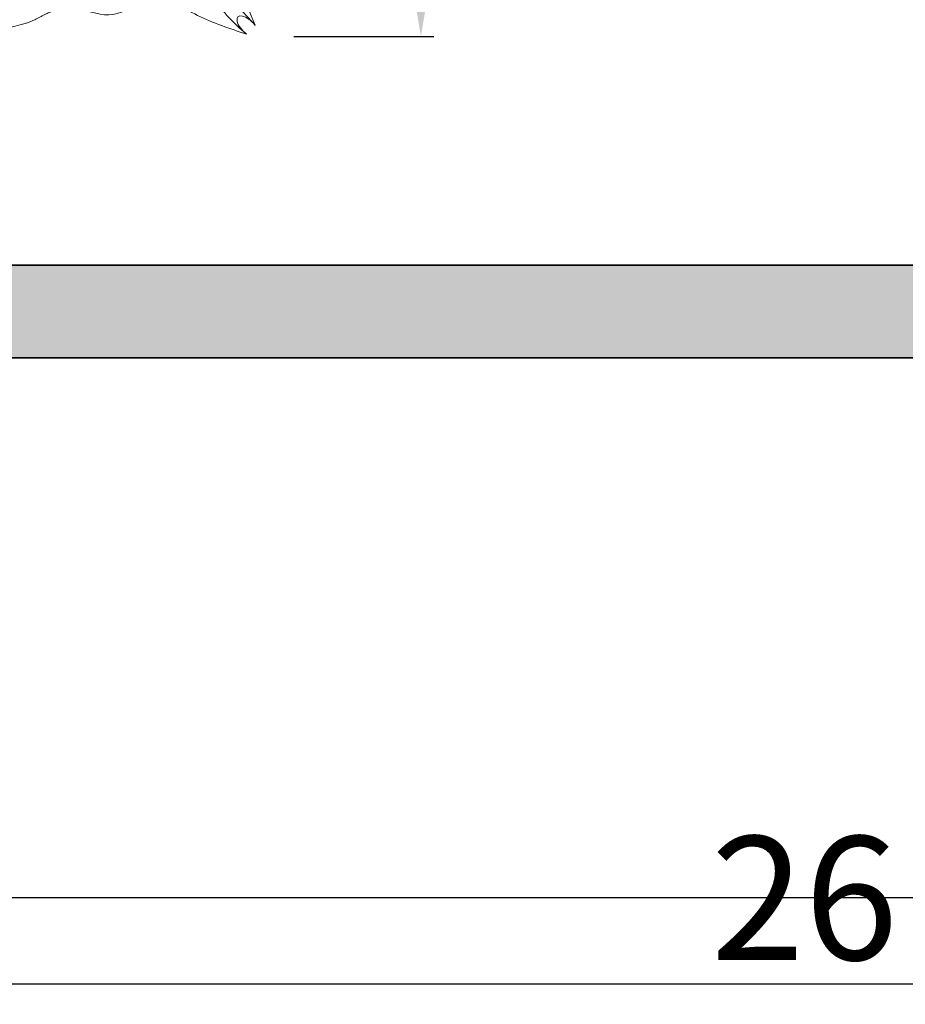
# Model space of a CAD drawing. Units: inches. Extents: x 2083 to 3317, y 1141 to 2115.
# Tile 3 of 256: x 2296 to 2382, y 1201 to 1296. Entities that reach past the tile are written whole.
import ezdxf

# ---------------------------------------------------------------- set-up
doc = ezdxf.new("R2010")
doc.units = ezdxf.units.IN
for name, color, linetype, lineweight in [('A-ANNO-DIMS', 2, 'Continuous', 18), ('A-FURN', 8, 'Continuous', 18), ('A-WALL', 7, 'Continuous', 35), ('www.cadblocksfree.com', 7, 'Continuous', 9)]:
    doc.layers.add(name, color=color, linetype=linetype, lineweight=lineweight)
doc.layers.add('A-WALL-PATT', color=251, linetype='Continuous', lineweight=13, true_color=0x636466)
doc.styles.get("Standard").update_dxf_attribs({"font": 'arial.ttf'})
doc.dimstyles.new('ISO-25', dxfattribs={"dimtxt": 12, "dimasz": 12, "dimexe": 1.25, "dimexo": 0.625, "dimtad": 1, "dimlunit": 3, "dimtxsty": 'Standard', "dimcen": 2.5, "dimadec": 0, "dimazin": 0, "dimtfac": 1, "dimtmove": 0, "dimatfit": 3, "dimfxl": 1, "dimarcsym": 0})

# ---------------------------------------------------------------- blocks, each defined once
blk = doc.blocks.new('bed')
at = {"layer": 'www.cadblocksfree.com', "ltscale": 0.2}
for centre, radius, start, end in [((3370.55, 1414.19), 11.47, 139.4648, 203.3712), ((3367.28, 1412.87), 7.94, 204.0179, 212.619)]:
    blk.add_arc(centre, radius, start, end, dxfattribs=at)
at = {"layer": 'www.cadblocksfree.com', "ltscale": 0.2, "extrusion": (0, 0, -1)}
for centre, major_axis, ratio, start_param, end_param in [((3360.34, 1388.37), (3.04, 3.04), 0.168252, 4.250342, 8.316029), ((3359.29, 1387.32), (1.05, 1.05), 0.453532, 4.422107, 8.144264)]:
    blk.add_ellipse(centre, major_axis=major_axis, ratio=ratio, start_param=start_param, end_param=end_param, dxfattribs=at)
at = {"layer": 'www.cadblocksfree.com', "ltscale": 0.2}
for points, knots in [([(3358.53, 1387.47), (3359.1, 1389.21), (3359.96, 1391.82), (3361.92, 1395.15), (3361.9, 1398.55), (3359.88, 1401.84), (3361.56, 1405.21), (3361.03, 1407.51), (3360.64, 1408.47), (3360.59, 1408.59)], [0, 0, 0, 0, 0.138875, 0.2092702, 0.2901949, 0.3858479, 0.4804923, 0.5489252, 0.5590752, 0.5590752, 0.5590752, 0.5590752]), ([(3430.32, 1386.56), (3427.33, 1387.65), (3422.15, 1389.55), (3414.53, 1384.14), (3405.61, 1387.05), (3396.29, 1386.31), (3386.84, 1381.28), (3377.74, 1390.27), (3370.78, 1384.8), (3364.63, 1383.97), (3363.28, 1388.27), (3360.78, 1387.15), (3359.45, 1386.56)], [0, 0, 0, 0, 8.93042, 15.449194, 25.485629, 34.878505, 43.598887, 54.554403, 64.16647, 67.461673, 70.610457, 74.213583, 74.213583, 74.213583, 74.213583])]:
    blk.add_open_spline(points, degree=3, knots=knots, dxfattribs=at)
blk = doc.blocks.new('*D12')
at = {"layer": 'A-ANNO-DIMS', "color": 0, "lineweight": -2, "transparency": 16777216}
for p, q in [((2226.96, 1262.636), (2226.96, 1201.284)), ((2544.96, 1262.636), (2544.96, 1201.284)), ((2238.96, 1202.534), (2532.96, 1202.534))]:
    blk.add_line(p, q, dxfattribs=at)
at = {"layer": 'A-ANNO-DIMS', "color": 0, "transparency": 16777216}
for points in [[(2238.96, 1204.534), (2238.96, 1200.534), (2226.96, 1202.534)], [(2532.96, 1204.534), (2532.96, 1200.534), (2544.96, 1202.534)]]:
    blk.add_solid(points, dxfattribs=at)
at = {"layer": 'Defpoints', "color": 0, "transparency": 16777216}
for p in [(2226.96, 1263.261), (2544.96, 1263.261), (2544.96, 1202.534)]:
    blk.add_point(p, dxfattribs=at)
at = {"layer": 'A-ANNO-DIMS', "color": 0, "transparency": 16777216, "insert": (2385.96, 1209.286), "char_height": 12, "attachment_point": 5}
blk.add_mtext('26\'-6"', dxfattribs=at)
blk = doc.blocks.new('*D23')
at = {"layer": 'A-ANNO-DIMS', "color": 0, "lineweight": -2, "transparency": 16777216}
for p, q in [((2335.205, 1362.114), (2335.205, 1476.472)), ((2322.885, 1362.114), (2336.455, 1362.114)), ((2335.205, 1306.473), (2335.205, 1350.114)), ((2322.885, 1294.473), (2336.455, 1294.473))]:
    blk.add_line(p, q, dxfattribs=at)
at = {"layer": 'A-ANNO-DIMS', "color": 0, "transparency": 16777216}
for points in [[(2333.205, 1350.114), (2337.205, 1350.114), (2335.205, 1362.114)], [(2333.205, 1306.473), (2337.205, 1306.473), (2335.205, 1294.473)]]:
    blk.add_solid(points, dxfattribs=at)
at = {"layer": 'Defpoints', "color": 0, "transparency": 16777216}
for p in [(2322.26, 1362.114), (2335.205, 1362.114), (2322.26, 1294.473)]:
    blk.add_point(p, dxfattribs=at)
at = {"layer": 'A-ANNO-DIMS', "color": 0, "transparency": 16777216, "insert": (2328.376, 1425.293), "char_height": 12, "attachment_point": 5, "rotation": 90}
blk.add_mtext('5\'-7 1/2" TYP.', dxfattribs=at)
blk = doc.blocks.new('*D34')
at = {"layer": 'A-ANNO-DIMS', "color": 0, "lineweight": -2, "transparency": 16777216}
for p, q in [((2226.96, 1262.636), (2226.96, 1209.661)), ((3126.96, 1262.636), (3126.96, 1209.661)), ((2238.96, 1210.911), (3114.96, 1210.911))]:
    blk.add_line(p, q, dxfattribs=at)
at = {"layer": 'A-ANNO-DIMS', "color": 0, "transparency": 16777216}
for points in [[(2238.96, 1212.911), (2238.96, 1208.911), (2226.96, 1210.911)], [(3114.96, 1212.911), (3114.96, 1208.911), (3126.96, 1210.911)]]:
    blk.add_solid(points, dxfattribs=at)
at = {"layer": 'Defpoints', "color": 0, "transparency": 16777216}
for p in [(2226.96, 1263.261), (3126.96, 1263.261), (3126.96, 1210.911)]:
    blk.add_point(p, dxfattribs=at)
at = {"layer": 'A-ANNO-DIMS', "color": 0, "transparency": 16777216, "insert": (2676.96, 1217.663), "char_height": 12, "attachment_point": 5}
blk.add_mtext('75\'-0"', dxfattribs=at)

msp = doc.modelspace()

# ---------------------------------------------------------------- hatches: boundary and pattern name
at = {"layer": 'A-WALL-PATT'}
h = msp.add_hatch(color=256, dxfattribs=at)
h.dxf.hatch_style = 1
h.paths.add_polyline_path([(3126.96, 2020.761), (2748.96, 2020.761), (2604.96, 2020.761), (2226.96, 2020.761), (2226.96, 1702.761), (2466.96, 1702.761), (2466.96, 1582.761), (2418.96, 1582.761), (2418.96, 1477.761), (2226.96, 1477.761), (2226.96, 1263.261), (2544.96, 1263.261), (2544.96, 1411.761), (2604.96, 1411.761), (2685.96, 1411.761), (2685.96, 1420.761), (2604.96, 1420.761), (2604.96, 1573.761), (2604.96, 1702.761), (2604.96, 2011.761), (2748.96, 2011.761), (2748.96, 1702.761), (2862.96, 1702.761), (2862.96, 1621.761), (2871.96, 1621.761), (2871.96, 1702.761), (2883.96, 1702.761), (2883.96, 1706.939, -0.026459), (2883.96, 1711.761), (2757.96, 1711.761), (2757.96, 1807.761), (2787.96, 1807.761), (2787.96, 1812.261), (2757.96, 1812.261), (2757.96, 2011.761), (2877.96, 2011.761), (2877.96, 1812.261), (2847.96, 1812.261), (2847.96, 1807.761), (2889.836, 1807.761), (2889.836, 1812.261), (2882.46, 1812.261), (2882.46, 2011.761), (3117.96, 2011.761), (3117.96, 1812.261), (2937.836, 1812.261), (2937.836, 1807.761), (2995.71, 1807.761), (2995.71, 1796.118), (3000.21, 1796.118), (3000.21, 1807.761), (3117.96, 1807.761), (3117.96, 1711.761), (3000.21, 1711.761), (3000.21, 1760.118), (2998.573, 1760.118, -0.020711), (2995.71, 1760.118), (2995.71, 1711.761), (2931.96, 1711.761), (2931.96, 1702.761), (3126.96, 1702.761)])
h.paths.add_polyline_path([(2471.46, 2011.761), (2471.46, 1810.011), (2462.717, 1810.011), (2462.717, 1805.511), (2505.96, 1805.511), (2505.96, 1810.011), (2475.96, 1810.011), (2475.96, 2011.761), (2595.96, 2011.761), (2595.96, 1810.011), (2565.96, 1810.011), (2565.96, 1805.511), (2595.96, 1805.511), (2595.96, 1711.761), (2235.96, 1711.761), (2235.96, 1805.511), (2353.71, 1805.511), (2353.71, 1796.054), (2358.21, 1796.054), (2358.21, 1805.511), (2414.717, 1805.511), (2414.717, 1810.011), (2235.96, 1810.011), (2235.96, 2011.761)], flags=16)
h.paths.add_polyline_path([(2270.205, 1994.61), (2270.205, 1970.61), (2246.205, 1970.61), (2246.205, 1994.61)], flags=0)
edge = h.paths.add_edge_path(flags=0)
edge.add_ellipse((2332.027, 1899.798), major_axis=(-3.043, 3.043), ratio=0.168252, start_angle=-161.33217, end_angle=-156.30711, ccw=False)
edge.add_ellipse((2333.082, 1898.744), major_axis=(-1.055, 1.055), ratio=0.453532, start_angle=-123.37102, end_angle=-94.15911)
edge = h.paths.add_edge_path(flags=0)
edge.add_ellipse((2332.027, 1968.876), major_axis=(3.043, 3.043), ratio=0.168252, start_angle=18.66783, end_angle=23.69289)
edge.add_spline(control_points=[(2332.926, 1970.691), (2332.227, 1970.336), (2330.894, 1969.659), (2328.413, 1970.932), (2327.204, 1967.749), (2324.71, 1969.956), (2322.533, 1967.012), (2320.013, 1971.296), (2317.68, 1968.158), (2316.041, 1967.102), (2315.427, 1966.81)], knot_values=[0, 0, 0, 0, 2.267059, 4.324559, 6.685584, 8.878641, 11.121502, 14.300359, 17.755284, 19.732645, 19.732645, 19.732645, 19.732645], degree=3, periodic=0)
edge.add_ellipse((2332.027, 1968.876), major_axis=(3.043, 3.043), ratio=0.168252, start_angle=18.66783, end_angle=23.69289, ccw=False)
edge.add_ellipse((2333.082, 1969.931), major_axis=(1.055, 1.055), ratio=0.453532, start_angle=56.62898, end_angle=85.84089, ccw=False)
edge = h.paths.add_edge_path(flags=0)
edge.add_spline(control_points=[(2296.428, 1967.988), (2293.628, 1965.336), (2287.704, 1959.727), (2299.744, 1949.996), (2294.533, 1935.669), (2290.573, 1920.604), (2293.394, 1909.974), (2296.185, 1904.967)], knot_values=[0.099185, 0.099185, 0.099185, 0.099185, 0.345301, 0.619822, 0.982653, 1.386093, 1.810555, 1.810555, 1.810555, 1.810555], degree=3, periodic=0)
edge.add_spline(control_points=[(2296.185, 1904.967), (2297.384, 1902.619), (2298.001, 1901.949), (2298.553, 1901.468)], knot_values=[0.006246, 0.006246, 0.006246, 0.006246, 0.055476, 0.055476, 0.055476, 0.055476], degree=3, periodic=0)
edge.add_spline(control_points=[(2298.553, 1901.468), (2297.259, 1900.923), (2295.225, 1900.232), (2293.06, 1900.614), (2292.101, 1900.788), (2292.09, 1900.791)], knot_values=[0.312835, 0.312835, 0.312835, 0.312835, 0.40178, 0.474987, 0.475903, 0.475903, 0.475903, 0.475903], degree=3, periodic=0)
edge.add_arc((2292.794, 1904.664), 3.937, 215.4209, 259.69818, ccw=False)
edge.add_spline(control_points=[(2289.585, 1902.382), (2289.477, 1902.535), (2289.368, 1902.688), (2289.261, 1902.841)], knot_values=[0.102872, 0.102872, 0.102872, 0.102872, 0.116896, 0.116896, 0.116896, 0.116896], degree=3, periodic=0)
edge.add_spline(control_points=[(2289.261, 1902.841), (2288.687, 1902.55), (2287.64, 1902.02), (2285.881, 1901.874), (2283.853, 1901.504), (2281.72, 1899.711), (2278.467, 1899.493), (2276.157, 1901.883), (2272.259, 1899.804), (2267.778, 1901.843), (2262.244, 1900.184), (2257.415, 1901.782), (2254.318, 1900.726), (2253.178, 1900.337)], knot_values=[0, 0, 0, 0, 1.907977, 3.477176, 5.261074, 7.972851, 11.680248, 13.717921, 16.939592, 22.789562, 27.502503, 33.595215, 37.145618, 37.145618, 37.145618, 37.145618], degree=3, periodic=0)
edge.add_line((2253.178, 1900.337), (2250.244, 1902.841))
edge.add_line((2250.244, 1902.841), (2250.244, 1965.833))
edge.add_line((2250.244, 1965.833), (2253.178, 1968.337))
edge.add_spline(control_points=[(2253.178, 1968.337), (2254.318, 1967.948), (2257.415, 1966.892), (2262.244, 1968.49), (2267.778, 1966.831), (2271.527, 1968.537), (2273.876, 1967.828), (2274.207, 1967.728)], knot_values=[0, 0, 0, 0, 0.09018, 0.244935, 0.364644, 0.513233, 0.537855, 0.537855, 0.537855, 0.537855], degree=3, periodic=0)
edge.add_arc((2274.353, 1963.793), 3.937, 72.05113, 92.12795, ccw=False)
edge.add_arc((2281.297, 1985.23), 18.596, 252.05113, 288.56572)
edge.add_arc((2292.317, 1956.029), 12.646, 71.02679, 113.77822, ccw=False)
edge = h.paths.add_edge_path(flags=0)
edge.add_spline(control_points=[(2274.899, 1951.856), (2275.066, 1951.617), (2275.233, 1951.377), (2275.398, 1951.136)], knot_values=[1.409916, 1.409916, 1.409916, 1.409916, 1.43159, 1.43159, 1.43159, 1.43159], degree=3, periodic=0)
edge.add_spline(control_points=[(2275.398, 1951.136), (2275.792, 1950.562), (2276.179, 1949.984), (2276.546, 1949.397)], knot_values=[1.358238, 1.358238, 1.358238, 1.358238, 1.409916, 1.409916, 1.409916, 1.409916], degree=3, periodic=0)
edge.add_line((2276.546, 1949.397), (2277.437, 1947.862))
edge.add_spline(control_points=[(2277.437, 1947.862), (2276.304, 1945.673), (2274.64, 1942.427), (2274.632, 1938.094), (2272.799, 1930.852), (2274.356, 1943.897), (2275.948, 1947.923), (2276.546, 1949.397)], knot_values=[0.005632, 0.005632, 0.005632, 0.005632, 0.186014, 0.266002, 0.357087, 0.59639, 0.739732, 0.739732, 0.739732, 0.739732], degree=3, periodic=0)
edge.add_spline(control_points=[(2276.546, 1949.397), (2276.179, 1949.984), (2275.792, 1950.562), (2275.398, 1951.136)], knot_values=[1.358238, 1.358238, 1.358238, 1.358238, 1.409916, 1.409916, 1.409916, 1.409916], degree=3, periodic=0)
edge.add_spline(control_points=[(2275.398, 1951.136), (2274.943, 1950.08), (2274.208, 1948.025), (2273.935, 1944.851), (2272.469, 1937.627), (2273.466, 1945.696), (2274.701, 1951.059), (2274.899, 1951.856)], knot_values=[0.104364, 0.104364, 0.104364, 0.104364, 0.189636, 0.269624, 0.36071, 0.600013, 0.644622, 0.644622, 0.644622, 0.644622], degree=3, periodic=0)
h.paths.add_polyline_path([(2269.168, 1963.128, -0.357527), (2268.171, 1960.976, -0.092561), (2268.171, 1939.436, -0.357527), (2269.168, 1937.285, -0.357527), (2267.016, 1938.282, -0.164785), (2254.686, 1938.282, -0.357527), (2252.534, 1937.285, -0.357527), (2253.531, 1939.436, -0.092561), (2253.531, 1960.976, -0.357527), (2252.534, 1963.128, -0.357527), (2254.686, 1962.131, -0.164785), (2267.016, 1962.131, -0.357527)], flags=0)
h.paths.add_polyline_path([(2248.874, 1967.802), (2248.874, 1957.028), (2249.458, 1957.028), (2249.458, 1911.647), (2248.874, 1911.647), (2248.874, 1900.873), (2246.512, 1900.873, 0.197327), (2244.15, 1902.457), (2244.15, 1966.218, 0.197327), (2246.512, 1967.802)], flags=0)
h.paths.add_polyline_path([(2269.168, 1931.389, -0.357527), (2268.171, 1929.238, -0.092561), (2268.171, 1907.698, -0.357527), (2269.168, 1905.547, -0.357527), (2267.016, 1906.544, -0.164785), (2254.686, 1906.544, -0.357527), (2252.534, 1905.547, -0.357527), (2253.531, 1907.698, -0.092561), (2253.531, 1929.238, -0.357527), (2252.534, 1931.389, -0.357527), (2254.686, 1930.392, -0.164785), (2267.016, 1930.392, -0.357527)], flags=0)
edge = h.paths.add_edge_path(flags=0)
edge.add_spline(control_points=[(2276.197, 1906.724), (2276.168, 1909.029), (2276.114, 1913.372), (2270.598, 1924.925), (2273.905, 1919.013), (2275.922, 1916.262), (2275.475, 1912.402), (2277.258, 1910.381), (2276.696, 1908.225), (2276.646, 1906.813), (2276.618, 1906.008)], knot_values=[0, 0, 0, 0, 8.61026, 16.221274, 18.843057, 23.804898, 27.440828, 29.356102, 31.203478, 33.650687, 33.650687, 33.650687, 33.650687], degree=3, periodic=0)
edge.add_spline(control_points=[(2276.618, 1906.008), (2276.623, 1905.624), (2276.498, 1904.629), (2275.442, 1903.855), (2274.937, 1903.08), (2274.859, 1902.841)], knot_values=[0.156488, 0.156488, 0.156488, 0.156488, 0.184398, 0.231376, 0.250598, 0.250598, 0.250598, 0.250598], degree=3, periodic=0)
edge.add_line((2274.859, 1902.841), (2276.506, 1902.841))
edge.add_spline(control_points=[(2276.506, 1902.841), (2276.788, 1903.085), (2277.665, 1904.125), (2278.25, 1904.341), (2277.654, 1908.527), (2278.156, 1906.228), (2278.1, 1905.286), (2278.847, 1904.069), (2277.857, 1903.415), (2277.874, 1902.991), (2277.904, 1902.841)], knot_values=[0.059574, 0.059574, 0.059574, 0.059574, 0.080753, 0.103741, 0.16972, 0.176036, 0.207137, 0.240474, 0.262341, 0.27366, 0.27366, 0.27366, 0.27366], degree=3, periodic=0)
edge.add_line((2277.904, 1902.841), (2280.03, 1902.841))
edge.add_spline(control_points=[(2280.03, 1902.841), (2279.888, 1903.088), (2279.499, 1903.982), (2280.152, 1905.939), (2278.104, 1909.658), (2279.762, 1907.185), (2280.328, 1904.875), (2280.485, 1903.49), (2281.463, 1903.249), (2281.758, 1902.936), (2281.834, 1902.841)], knot_values=[0.013856, 0.013856, 0.013856, 0.013856, 0.034874, 0.088867, 0.107879, 0.126738, 0.158714, 0.193757, 0.217487, 0.226722, 0.226722, 0.226722, 0.226722], degree=3, periodic=0)
edge.add_spline(control_points=[(2281.834, 1902.841), (2281.788, 1902.827), (2281.647, 1902.783), (2281.396, 1902.859), (2281.088, 1902.985), (2280.721, 1903.061), (2280.333, 1903.026), (2280.125, 1902.899), (2280.03, 1902.841)], knot_values=[0, 0, 0, 0, 0.14413, 0.435517, 0.749276, 1.153046, 1.548371, 1.878348, 1.878348, 1.878348, 1.878348], degree=3, periodic=0)
edge.add_line((2280.03, 1902.841), (2277.904, 1902.841))
edge.add_spline(control_points=[(2277.904, 1902.841), (2277.893, 1902.796), (2277.865, 1902.68), (2277.607, 1902.687), (2277.274, 1902.801), (2276.838, 1902.62), (2276.584, 1902.789), (2276.506, 1902.841)], knot_values=[0, 0, 0, 0, 0.127189, 0.326199, 0.628009, 1.24357, 1.515331, 1.515331, 1.515331, 1.515331], degree=3, periodic=0)
edge.add_line((2276.506, 1902.841), (2274.859, 1902.841))
edge.add_spline(control_points=[(2274.859, 1902.841), (2274.814, 1902.899), (2274.725, 1903.013), (2274.493, 1903.119), (2274.244, 1902.961), (2273.937, 1903.185), (2273.614, 1902.983), (2273.408, 1902.883), (2273.322, 1902.841)], knot_values=[0, 0, 0, 0, 0.21843, 0.436957, 0.687977, 0.990379, 1.398396, 1.69185, 1.69185, 1.69185, 1.69185], degree=3, periodic=0)
edge.add_spline(control_points=[(2273.322, 1902.841), (2273.617, 1903.446), (2274.274, 1904.538), (2276.027, 1904.574), (2276.207, 1906.584), (2276.197, 1906.724)], knot_values=[0.012227, 0.012227, 0.012227, 0.012227, 0.059472, 0.106218, 0.134458, 0.134458, 0.134458, 0.134458], degree=3, periodic=0)
h.paths.add_polyline_path([(2270.776, 1897.79), (2270.776, 1873.79), (2246.776, 1873.79), (2246.776, 1897.79)], flags=0)
h.paths.add_polyline_path([(2353.71, 1760.005), (2353.71, 1760.054), (2358.21, 1760.054, -0.033729)], flags=0)
h.paths.add_polyline_path([(2321.819, 1737.529), (2341.995, 1737.529, -0.414214), (2343.203, 1736.321), (2343.203, 1721.021, -0.414214), (2341.995, 1719.813), (2321.819, 1719.813, -0.414214), (2320.611, 1721.021), (2320.611, 1736.321, -0.414214)], flags=0)
h.paths.add_polyline_path([(2324.235, 1736.321), (2339.579, 1736.321, -0.414214), (2341.995, 1733.905), (2341.995, 1725.45, -0.414214), (2339.579, 1723.034), (2333.681, 1723.034), (2333.845, 1722.045, -0.870646), (2335.425, 1721.826, -0.767327), (2333.923, 1721.423), (2331.291, 1721.423, -0.767327), (2329.788, 1721.826, -0.870646), (2331.368, 1722.045), (2331.533, 1723.034), (2324.235, 1723.034, -0.414214), (2321.819, 1725.45), (2321.819, 1733.905, -0.414214)], flags=0)
h.paths.add_polyline_path([(2570.484, 1928.615), (2589.684, 1928.615), (2590.169, 1928.615), (2590.169, 1904.993), (2570.484, 1904.993)], flags=0)
h.paths.add_polyline_path([(2574.447, 1927.264, -1), (2572.829, 1927.264, -1)], flags=0)
h.paths.add_polyline_path([(2573.09, 1926.941), (2573.925, 1927.776), (2574.148, 1927.553), (2573.313, 1926.718)], flags=0)
h.paths.add_polyline_path([(2578.779, 1919.73, -1), (2571.592, 1919.73, -1)], flags=0)
h.paths.add_polyline_path([(2578.385, 1919.73, -1), (2571.985, 1919.73, -1)], flags=0)
h.paths.add_polyline_path([(2331.596, 1729.476, -1), (2333.618, 1729.476, -1)], flags=0)
h.paths.add_polyline_path([(2578.034, 1927.264, -1), (2576.416, 1927.264, -1)], flags=0)
h.paths.add_polyline_path([(2576.689, 1927.531), (2576.912, 1927.754), (2577.747, 1926.919), (2577.524, 1926.696)], flags=0)
h.paths.add_polyline_path([(2578.139, 1909.86, -1), (2572.232, 1909.86, -1)], flags=0)
h.paths.add_polyline_path([(2577.745, 1909.86, -1), (2572.625, 1909.86, -1)], flags=0)
h.paths.add_polyline_path([(2583.798, 1927.264, -1), (2582.179, 1927.264, -1)], flags=0)
h.paths.add_polyline_path([(2582.719, 1927.754), (2583.554, 1926.919), (2583.331, 1926.696), (2582.496, 1927.531)], flags=0)
h.paths.add_polyline_path([(2582.496, 1927.531), (2582.719, 1927.754), (2583.554, 1926.919), (2583.331, 1926.696)], flags=0)
h.paths.add_polyline_path([(2587.739, 1920.53, -1), (2581.832, 1920.53, -1)], flags=0)
h.paths.add_polyline_path([(2587.345, 1920.53, -1), (2582.225, 1920.53, -1)], flags=0)
h.paths.add_polyline_path([(2587.385, 1927.264, -1), (2585.766, 1927.264, -1)], flags=0)
h.paths.add_polyline_path([(2586.082, 1926.98), (2586.917, 1927.815), (2587.14, 1927.593), (2586.305, 1926.758)], flags=0)
h.paths.add_polyline_path([(2588.379, 1910.66, -1), (2581.192, 1910.66, -1)], flags=0)
h.paths.add_polyline_path([(2587.985, 1910.66, -1), (2581.585, 1910.66, -1)], flags=0)
h.paths.add_polyline_path([(2417.168, 1729.478), (2437.344, 1729.478, -0.414214), (2438.552, 1728.27), (2438.552, 1712.969, -0.414214), (2437.344, 1711.761), (2417.168, 1711.761, -0.414214), (2415.96, 1712.969), (2415.96, 1728.27, -0.414214)], flags=0)
h.paths.add_polyline_path([(2419.584, 1728.27), (2434.928, 1728.27, -0.414214), (2437.344, 1725.854), (2437.344, 1717.398, -0.414214), (2434.928, 1714.983), (2429.029, 1714.983), (2429.194, 1713.994, -0.870646), (2430.774, 1713.775, -0.767327), (2429.271, 1713.372), (2426.64, 1713.372, -0.767327), (2425.137, 1713.775, -0.870646), (2426.717, 1713.994), (2426.882, 1714.983), (2419.584, 1714.983, -0.414214), (2417.168, 1717.398), (2417.168, 1725.854, -0.414214)], flags=0)
h.paths.add_polyline_path([(2419.584, 1728.27), (2434.928, 1728.27, -0.414214), (2437.344, 1725.854), (2437.344, 1717.398, -0.414214), (2434.928, 1714.983), (2429.029, 1714.983), (2428.358, 1719.009), (2427.553, 1719.009), (2426.882, 1714.983), (2419.584, 1714.983, -0.414214), (2417.168, 1717.398), (2417.168, 1725.854, -0.414214)], flags=0)
h.paths.add_polyline_path([(2426.944, 1721.425, -1), (2428.967, 1721.425, -1)], flags=0)
h.paths.add_polyline_path([(2475.96, 1702.761), (2595.96, 1702.761), (2595.96, 1582.761), (2475.96, 1582.761)], flags=16)
h.paths.add_polyline_path([(2427.96, 1573.761), (2595.96, 1573.761), (2595.96, 1468.761), (2595.96, 1420.761), (2384.46, 1420.761), (2384.46, 1468.761), (2427.96, 1468.761)], flags=16)
h.paths.add_polyline_path([(2379.96, 1468.761), (2379.96, 1420.761), (2235.96, 1420.761), (2235.96, 1468.761)], flags=16)
h.paths.add_polyline_path([(2317.816, 1466.696), (2337.992, 1466.696, -0.414214), (2339.2, 1465.488), (2339.2, 1450.187, -0.414214), (2337.992, 1448.979), (2317.816, 1448.979, -0.414214), (2316.608, 1450.187), (2316.608, 1465.488, -0.414214)], flags=0)
h.paths.add_polyline_path([(2320.232, 1465.488), (2335.576, 1465.488, -0.414214), (2337.992, 1463.072), (2337.992, 1454.616, -0.414214), (2335.576, 1452.2), (2329.677, 1452.2), (2329.842, 1451.212, -0.870646), (2331.422, 1450.992, -0.767327), (2329.92, 1450.59), (2327.288, 1450.59, -0.767327), (2325.785, 1450.992, -0.870646), (2327.365, 1451.212), (2327.53, 1452.2), (2320.232, 1452.2, -0.414214), (2317.816, 1454.616), (2317.816, 1463.072, -0.414214)], flags=0)
h.paths.add_polyline_path([(2320.232, 1465.488), (2335.576, 1465.488, -0.414214), (2337.992, 1463.072), (2337.992, 1454.616, -0.414214), (2335.576, 1452.2), (2329.677, 1452.2), (2329.006, 1456.227), (2328.201, 1456.227), (2327.53, 1452.2), (2320.232, 1452.2, -0.414214), (2317.816, 1454.616), (2317.816, 1463.072, -0.414214)], flags=0)
h.paths.add_polyline_path([(2327.593, 1458.643, -1), (2329.615, 1458.643, -1)], flags=0)
h.paths.add_polyline_path([(2244.412, 1433.34), (2241.921, 1433.34, -0.414214), (2240.018, 1435.244), (2240.018, 1440.953, -0.414211), (2241.921, 1442.856), (2244.412, 1442.856, -1.976472)], flags=0)
h.paths.add_polyline_path([(2245.357, 1434.398, -0.414214), (2245.357, 1441.799, -2.144098)], flags=0)
h.paths.add_polyline_path([(2535.96, 1416.261), (2535.96, 1272.261), (2235.96, 1272.261), (2235.96, 1416.261)], flags=16)
h.paths.add_polyline_path([(2260.12, 1384.293), (2260.12, 1362.039), (2237.865, 1362.039), (2237.865, 1384.293)], flags=0)
edge = h.paths.add_edge_path(flags=0)
edge.add_line((2318.252, 1362.093), (2318.146, 1362.001))
edge.add_ellipse((2317.445, 1360.431), major_axis=(2.822, 2.822), ratio=0.168252, start_angle=18.66783, end_angle=20.94813, ccw=False)
edge.add_ellipse((2318.423, 1361.409), major_axis=(0.978, 0.978), ratio=0.453532, start_angle=56.62898, end_angle=70.2262, ccw=False)
edge = h.paths.add_edge_path(flags=0)
edge.add_line((2319.107, 1295.571), (2319.015, 1295.677))
edge.add_ellipse((2317.445, 1296.378), major_axis=(-2.822, 2.822), ratio=0.168252, start_angle=-161.33217, end_angle=-159.05187, ccw=False)
edge.add_ellipse((2318.423, 1295.4), major_axis=(-0.978, 0.978), ratio=0.453532, start_angle=-123.37102, end_angle=-109.7738)
edge = h.paths.add_edge_path(flags=0)
edge.add_spline(control_points=[(2284.21, 1301.17), (2284.581, 1300.445), (2284.891, 1299.892), (2285.16, 1299.461)], knot_values=[0.039066, 0.039066, 0.039066, 0.039066, 0.055476, 0.055476, 0.055476, 0.055476], degree=3, periodic=0)
edge.add_line((2285.16, 1299.461), (2284.21, 1301.17))
edge = h.paths.add_edge_path(flags=0)
edge.add_line((2280.412, 1297.298), (2283.37, 1297.036))
edge.add_line((2283.37, 1297.036), (2286.406, 1297.926))
edge.add_spline(control_points=[(2286.406, 1297.926), (2285.305, 1297.463), (2284.345, 1297.129), (2283.37, 1297.036)], knot_values=[0.394369, 0.394369, 0.394369, 0.394369, 0.475903, 0.475903, 0.475903, 0.475903], degree=3, periodic=0)
edge.add_spline(control_points=[(2283.37, 1297.036), (2283.281, 1297.028), (2282.316, 1296.957), (2281.313, 1297.134), (2280.423, 1297.296), (2280.412, 1297.298)], knot_values=[0.312835, 0.312835, 0.312835, 0.312835, 0.320246, 0.393453, 0.394369, 0.394369, 0.394369, 0.394369], degree=3, periodic=0)
edge = h.paths.add_edge_path(flags=0)
edge.add_line((2284.436, 1359.607), (2280.446, 1355.328))
edge.add_line((2280.446, 1355.328), (2279.58, 1351.018))
edge.add_line((2279.58, 1351.018), (2282.413, 1346.58))
edge.add_spline(control_points=[(2282.413, 1346.58), (2283.153, 1345.589), (2284.253, 1344.029), (2284.801, 1342.387), (2284.935, 1341.806)], knot_values=[1.240098, 1.240098, 1.240098, 1.240098, 1.332892, 1.382712, 1.382712, 1.382712, 1.382712], degree=3, periodic=0)
edge.add_spline(control_points=[(2284.935, 1341.806), (2285.319, 1340.141), (2285.233, 1338.409), (2284.91, 1336.654)], knot_values=[1.097484, 1.097484, 1.097484, 1.097484, 1.240098, 1.240098, 1.240098, 1.240098], degree=3, periodic=0)
edge.add_spline(control_points=[(2284.91, 1336.654), (2284.587, 1334.899), (2284.027, 1333.12), (2283.463, 1331.361)], knot_values=[0.95487, 0.95487, 0.95487, 0.95487, 1.097484, 1.097484, 1.097484, 1.097484], degree=3, periodic=0)
edge.add_line((2283.463, 1331.361), (2281.89, 1326.153))
edge.add_line((2281.89, 1326.153), (2280.756, 1321.056))
edge.add_line((2280.756, 1321.056), (2280.299, 1316.002))
edge.add_line((2280.299, 1316.002), (2280.716, 1310.95))
edge.add_line((2280.716, 1310.95), (2282.028, 1305.972))
edge.add_line((2282.028, 1305.972), (2284.21, 1301.17))
edge.add_spline(control_points=[(2284.21, 1301.17), (2283.341, 1302.73), (2282.612, 1304.336), (2282.028, 1305.972)], knot_values=[0.099185, 0.099185, 0.099185, 0.099185, 0.241799, 0.241799, 0.241799, 0.241799], degree=3, periodic=0)
edge.add_spline(control_points=[(2282.028, 1305.972), (2281.444, 1307.608), (2281.005, 1309.273), (2280.716, 1310.95)], knot_values=[0.241799, 0.241799, 0.241799, 0.241799, 0.384413, 0.384413, 0.384413, 0.384413], degree=3, periodic=0)
edge.add_spline(control_points=[(2280.716, 1310.95), (2280.433, 1312.588), (2280.289, 1314.277), (2280.299, 1315.962), (2280.299, 1316.002)], knot_values=[0.384413, 0.384413, 0.384413, 0.384413, 0.523647, 0.527028, 0.527028, 0.527028, 0.527028], degree=3, periodic=0)
edge.add_spline(control_points=[(2280.299, 1316.002), (2280.312, 1317.687), (2280.478, 1319.368), (2280.756, 1321.056)], knot_values=[0.527028, 0.527028, 0.527028, 0.527028, 0.669642, 0.669642, 0.669642, 0.669642], degree=3, periodic=0)
edge.add_spline(control_points=[(2280.756, 1321.056), (2281.035, 1322.744), (2281.426, 1324.44), (2281.89, 1326.153)], knot_values=[0.669642, 0.669642, 0.669642, 0.669642, 0.812256, 0.812256, 0.812256, 0.812256], degree=3, periodic=0)
edge.add_spline(control_points=[(2281.89, 1326.153), (2282.264, 1327.533), (2282.788, 1329.262), (2283.353, 1331.018), (2283.463, 1331.361)], knot_values=[0.812256, 0.812256, 0.812256, 0.812256, 0.927087, 0.95487, 0.95487, 0.95487, 0.95487], degree=3, periodic=0)
edge.add_line((2283.463, 1331.361), (2284.91, 1336.654))
edge.add_line((2284.91, 1336.654), (2284.935, 1341.806))
edge.add_line((2284.935, 1341.806), (2282.413, 1346.58))
edge.add_spline(control_points=[(2282.413, 1346.58), (2281.275, 1348.104), (2280.078, 1349.57), (2279.58, 1351.018)], knot_values=[1.382712, 1.382712, 1.382712, 1.382712, 1.525326, 1.525326, 1.525326, 1.525326], degree=3, periodic=0)
edge.add_spline(control_points=[(2279.58, 1351.018), (2279.443, 1351.415), (2279.136, 1352.857), (2279.735, 1354.29), (2280.446, 1355.328)], knot_values=[1.525326, 1.525326, 1.525326, 1.525326, 1.564439, 1.667941, 1.667941, 1.667941, 1.667941], degree=3, periodic=0)
edge.add_spline(control_points=[(2280.446, 1355.328), (2281.426, 1356.758), (2282.931, 1358.183), (2284.436, 1359.607)], knot_values=[1.667941, 1.667941, 1.667941, 1.667941, 1.810555, 1.810555, 1.810555, 1.810555], degree=3, periodic=0)
edge.add_arc((2280.623, 1348.518), 11.726, 71.02679, 113.77822)
edge.add_arc((2270.405, 1375.595), 17.244, 252.05113, 288.56572, ccw=False)
edge.add_arc((2263.966, 1355.718), 3.651, 72.05113, 92.12795)
edge.add_arc((2263.966, 1355.718), 3.651, 92.12795, 177.98513)
edge.add_spline(control_points=[(2260.318, 1355.846), (2260.26, 1354.221), (2260.551, 1350.187), (2262.999, 1346.766), (2264.473, 1344.649)], knot_values=[1.43159, 1.43159, 1.43159, 1.43159, 1.564144, 1.770695, 1.770695, 1.770695, 1.770695], degree=3, periodic=0)
edge.add_line((2264.473, 1344.649), (2264.936, 1343.983))
edge.add_spline(control_points=[(2263.801, 1340.248), (2263.843, 1340.514), (2264.067, 1341.756), (2264.513, 1343.002), (2264.935, 1343.981)], knot_values=[0.53657, 0.53657, 0.53657, 0.53657, 0.559349, 0.644622, 0.644622, 0.644622, 0.644622], degree=3, periodic=0)
edge.add_spline(control_points=[(2264.935, 1343.981), (2265.118, 1343.715), (2265.299, 1343.448), (2265.477, 1343.179)], knot_values=[1.384077, 1.384077, 1.384077, 1.384077, 1.409916, 1.409916, 1.409916, 1.409916], degree=3, periodic=0)
edge.add_spline(control_points=[(2265.477, 1343.179), (2265.655, 1342.911), (2265.829, 1342.641), (2265.999, 1342.369)], knot_values=[1.358238, 1.358238, 1.358238, 1.358238, 1.384077, 1.384077, 1.384077, 1.384077], degree=3, periodic=0)
edge.add_line((2265.999, 1342.369), (2266.826, 1340.946))
edge.add_spline(control_points=[(2266.826, 1340.946), (2268.894, 1337.09), (2271.398, 1325.843), (2270.516, 1310.569), (2275.919, 1301.861), (2277.79, 1299.199)], knot_values=[0.116896, 0.116896, 0.116896, 0.116896, 0.472987, 1.050969, 1.313793, 1.313793, 1.313793, 1.313793], degree=3, periodic=0)
edge.add_spline(control_points=[(2277.79, 1299.199), (2277.839, 1299.128), (2277.889, 1299.057), (2277.94, 1298.987)], knot_values=[0.109884, 0.109884, 0.109884, 0.109884, 0.116896, 0.116896, 0.116896, 0.116896], degree=3, periodic=0)
edge.add_line((2277.94, 1298.987), (2277.789, 1299.199))
edge.add_spline(control_points=[(2277.789, 1299.199), (2277.257, 1298.929), (2276.286, 1298.438), (2275.039, 1298.334), (2274.383, 1298.239), (2274.215, 1298.209)], knot_values=[33.12187, 33.12187, 33.12187, 33.12187, 35.029056, 36.598255, 37.144827, 37.144827, 37.144827, 37.144827], degree=3, periodic=0)
edge.add_line((2274.215, 1298.209), (2273.073, 1297.893))
edge.add_spline(control_points=[(2273.073, 1297.893), (2272.323, 1297.58), (2271.039, 1296.511), (2269.248, 1296.226), (2268.423, 1296.375)], knot_values=[26.532584, 26.532584, 26.532584, 26.532584, 29.198919, 31.839101, 31.839101, 31.839101, 31.839101], degree=3, periodic=0)
edge.add_line((2268.423, 1296.375), (2263.879, 1297.458))
edge.add_spline(control_points=[(2263.879, 1297.458), (2263.556, 1297.359), (2261.86, 1296.839), (2260.239, 1297.282), (2258.933, 1297.516)], knot_values=[15.919551, 15.919551, 15.919551, 15.919551, 16.939592, 21.226067, 21.226067, 21.226067, 21.226067], degree=3, periodic=0)
edge.add_line((2258.933, 1297.516), (2254.055, 1297.329))
edge.add_spline(control_points=[(2254.055, 1297.329), (2253.756, 1297.296), (2252.114, 1297.165), (2250.462, 1297.544), (2249.13, 1297.668)], knot_values=[5.306517, 5.306517, 5.306517, 5.306517, 6.276435, 10.613034, 10.613034, 10.613034, 10.613034], degree=3, periodic=0)
edge.add_line((2249.13, 1297.668), (2244.332, 1296.878))
edge.add_line((2244.332, 1296.878), (2241.611, 1299.199))
edge.add_line((2241.611, 1299.199), (2241.611, 1357.609))
edge.add_line((2241.611, 1357.609), (2244.332, 1359.931))
edge.add_line((2244.332, 1359.931), (2252.729, 1359.543))
edge.add_spline(control_points=[(2252.729, 1359.543), (2252.871, 1359.546), (2253.306, 1359.548), (2253.74, 1359.514), (2254.032, 1359.482)], knot_values=[0.233291, 0.233291, 0.233291, 0.233291, 0.244935, 0.268927, 0.268927, 0.268927, 0.268927], degree=3, periodic=0)
edge.add_line((2254.032, 1359.482), (2259.587, 1359.416))
edge.add_spline(control_points=[(2259.587, 1359.416), (2260.677, 1359.629), (2262.073, 1359.897), (2263.524, 1359.459), (2263.83, 1359.366)], knot_values=[0.422516, 0.422516, 0.422516, 0.422516, 0.513233, 0.537855, 0.537855, 0.537855, 0.537855], degree=3, periodic=0)
edge.add_arc((2263.966, 1355.718), 3.651, 72.05113, 92.12795, ccw=False)
edge.add_arc((2270.405, 1375.595), 17.244, 252.05113, 288.56572)
edge.add_arc((2280.623, 1348.518), 11.726, 71.02679, 113.77822, ccw=False)
h.paths.add_polyline_path([(2240.341, 1359.435), (2240.341, 1349.444), (2240.882, 1349.444), (2240.882, 1307.365), (2240.341, 1307.365), (2240.341, 1297.374), (2238.15, 1297.374, 0.197327), (2235.96, 1298.843), (2235.96, 1357.966, 0.197327), (2238.15, 1359.435)], flags=0)
h.paths.add_polyline_path([(2259.158, 1355.101, -0.357527), (2258.233, 1353.106, -0.092561), (2258.233, 1333.133, -0.357527), (2259.158, 1331.138, -0.357527), (2257.163, 1332.062, -0.164785), (2245.729, 1332.062, -0.357527), (2243.735, 1331.138, -0.357527), (2244.659, 1333.133, -0.092561), (2244.659, 1353.106, -0.357527), (2243.735, 1355.101, -0.357527), (2245.729, 1354.176, -0.164785), (2257.163, 1354.176, -0.357527)], flags=0)
edge = h.paths.add_edge_path(flags=0)
edge.add_line((2265.999, 1342.369), (2266.826, 1340.946))
edge.add_line((2266.826, 1340.946), (2265.308, 1337.814))
edge.add_line((2265.308, 1337.814), (2264.358, 1334.653))
edge.add_line((2264.358, 1334.653), (2264.262, 1333.8))
edge.add_spline(control_points=[(2264.262, 1333.8), (2264.208, 1333.187), (2264.162, 1332.366), (2264.007, 1331.414), (2263.969, 1331.202)], knot_values=[0.464444, 0.464444, 0.464444, 0.464444, 0.516691, 0.531608, 0.531608, 0.531608, 0.531608], degree=3, periodic=0)
edge.add_spline(control_points=[(2263.969, 1331.202), (2263.775, 1330.119), (2263.424, 1328.791), (2263.257, 1328.531), (2263.234, 1328.515)], knot_values=[0.372682, 0.372682, 0.372682, 0.372682, 0.44885, 0.464444, 0.464444, 0.464444, 0.464444], degree=3, periodic=0)
edge.add_spline(control_points=[(2263.234, 1328.515), (2263.096, 1328.42), (2263.131, 1329.301), (2263.275, 1330.616)], knot_values=[0.280919, 0.280919, 0.280919, 0.280919, 0.372682, 0.372682, 0.372682, 0.372682], degree=3, periodic=0)
edge.add_spline(control_points=[(2263.275, 1330.616), (2263.419, 1331.93), (2263.672, 1333.677), (2263.97, 1335.315)], knot_values=[0.189157, 0.189157, 0.189157, 0.189157, 0.280919, 0.280919, 0.280919, 0.280919], degree=3, periodic=0)
edge.add_spline(control_points=[(2263.97, 1335.315), (2264.1, 1336.032), (2264.419, 1337.622), (2264.755, 1338.864), (2264.947, 1339.491)], knot_values=[0.097394, 0.097394, 0.097394, 0.097394, 0.137578, 0.189157, 0.189157, 0.189157, 0.189157], degree=3, periodic=0)
edge.add_spline(control_points=[(2264.947, 1339.491), (2265.29, 1340.606), (2265.644, 1341.494), (2265.999, 1342.369)], knot_values=[0.005632, 0.005632, 0.005632, 0.005632, 0.097394, 0.097394, 0.097394, 0.097394], degree=3, periodic=0)
h.paths.add_polyline_path([(2259.158, 1325.671, -0.357527), (2258.233, 1323.676, -0.092561), (2258.233, 1303.703, -0.357527), (2259.158, 1301.708, -0.357527), (2257.163, 1302.633, -0.164785), (2245.729, 1302.633, -0.357527), (2243.735, 1301.708, -0.357527), (2244.659, 1303.703, -0.092561), (2244.659, 1323.676, -0.357527), (2243.735, 1325.671, -0.357527), (2245.729, 1324.747, -0.164785), (2257.163, 1324.747, -0.357527)], flags=0)
edge = h.paths.add_edge_path(flags=0)
edge.add_spline(control_points=[(2261.709, 1317.311), (2261.679, 1317.418), (2261.762, 1317.389), (2262.491, 1316.09), (2262.962, 1315.301)], knot_values=[14.955861, 14.955861, 14.955861, 14.955861, 16.221274, 18.694826, 18.694826, 18.694826, 18.694826], degree=3, periodic=0)
edge.add_spline(control_points=[(2262.962, 1315.301), (2262.99, 1315.254), (2263.702, 1314.067), (2264.349, 1313.127), (2264.73, 1312.164)], knot_values=[18.694826, 18.694826, 18.694826, 18.694826, 18.843057, 22.433791, 22.433791, 22.433791, 22.433791], degree=3, periodic=0)
edge.add_spline(control_points=[(2264.73, 1312.164), (2264.876, 1311.796), (2265.177, 1310.77), (2265.143, 1309.559), (2265.248, 1308.824)], knot_values=[22.433791, 22.433791, 22.433791, 22.433791, 23.804898, 26.172756, 26.172756, 26.172756, 26.172756], degree=3, periodic=0)
edge.add_line((2265.248, 1308.824), (2265.851, 1307.172))
edge.add_spline(control_points=[(2265.851, 1307.172), (2266.065, 1306.822), (2266.384, 1306.332), (2266.424, 1305.781), (2266.42, 1305.611)], knot_values=[28.062562, 28.062562, 28.062562, 28.062562, 29.356102, 29.911721, 29.911721, 29.911721, 29.911721], degree=3, periodic=0)
edge.add_spline(control_points=[(2266.42, 1305.611), (2266.416, 1305.433), (2266.394, 1305.25), (2266.365, 1305.066)], knot_values=[29.911721, 29.911721, 29.911721, 29.911721, 30.497837, 30.497837, 30.497837, 30.497837], degree=3, periodic=0)
edge.add_line((2266.365, 1305.066), (2266.066, 1302.136))
edge.add_spline(control_points=[(2266.066, 1302.136), (2266.071, 1301.78), (2265.998, 1301.2), (2265.663, 1300.759), (2265.509, 1300.586)], knot_values=[0.156488, 0.156488, 0.156488, 0.156488, 0.184398, 0.203543, 0.203543, 0.203543, 0.203543], degree=3, periodic=0)
edge.add_line((2265.509, 1300.586), (2264.435, 1299.199))
edge.add_line((2264.435, 1299.199), (2265.962, 1299.199))
edge.add_line((2265.962, 1299.199), (2267.336, 1301.175))
edge.add_line((2267.336, 1301.175), (2267.312, 1301.986))
edge.add_spline(control_points=[(2267.312, 1301.986), (2267.261, 1302.862), (2267.16, 1303.737), (2267.271, 1303.326)], knot_values=[0.126229, 0.126229, 0.126229, 0.126229, 0.166617, 0.166617, 0.166617, 0.166617], degree=3, periodic=0)
edge.add_spline(control_points=[(2267.271, 1303.326), (2267.28, 1303.294), (2267.31, 1303.175), (2267.373, 1302.884), (2267.406, 1302.683), (2267.418, 1302.601)], knot_values=[0.166617, 0.166617, 0.166617, 0.166617, 0.16972, 0.176036, 0.180765, 0.180765, 0.180765, 0.180765], degree=3, periodic=0)
edge.add_spline(control_points=[(2267.744, 1300.988), (2267.688, 1301.151), (2267.481, 1301.657), (2267.484, 1302.145), (2267.418, 1302.601)], knot_values=[0.180765, 0.180765, 0.180765, 0.180765, 0.193767, 0.220139, 0.220139, 0.220139, 0.220139], degree=3, periodic=0)
edge.add_line((2267.418, 1302.601), (2267.744, 1300.988))
edge.add_spline(control_points=[(2267.744, 1300.988), (2267.832, 1300.732), (2267.932, 1300.31), (2267.555, 1299.975), (2267.429, 1299.829)], knot_values=[0.220139, 0.220139, 0.220139, 0.220139, 0.240474, 0.25489, 0.25489, 0.25489, 0.25489], degree=3, periodic=0)
edge.add_line((2267.429, 1299.829), (2267.258, 1299.199))
edge.add_line((2267.258, 1299.199), (2269.23, 1299.199))
edge.add_spline(control_points=[(2269.23, 1299.199), (2269.099, 1299.429), (2268.843, 1300.016), (2269.012, 1300.916), (2268.947, 1301.661)], knot_values=[0.013856, 0.013856, 0.013856, 0.013856, 0.034874, 0.067073, 0.067073, 0.067073, 0.067073], degree=3, periodic=0)
edge.add_line((2268.947, 1301.661), (2268.432, 1303.603))
edge.add_spline(control_points=[(2268.432, 1303.603), (2268.176, 1304.192), (2267.596, 1305.251), (2268.041, 1304.623), (2268.251, 1304.282)], knot_values=[0.090155, 0.090155, 0.090155, 0.090155, 0.107879, 0.120289, 0.120289, 0.120289, 0.120289], degree=3, periodic=0)
edge.add_spline(control_points=[(2268.251, 1304.282), (2268.361, 1304.105), (2269.058, 1302.918), (2269.383, 1301.59), (2269.521, 1300.776), (2269.575, 1300.556)], knot_values=[0.120289, 0.120289, 0.120289, 0.120289, 0.126738, 0.158714, 0.173506, 0.173506, 0.173506, 0.173506], degree=3, periodic=0)
edge.add_line((2269.575, 1300.556), (2270.686, 1299.421))
edge.add_spline(control_points=[(2270.686, 1299.421), (2270.767, 1299.357), (2270.838, 1299.281), (2270.903, 1299.199)], knot_values=[0.21816, 0.21816, 0.21816, 0.21816, 0.226722, 0.226722, 0.226722, 0.226722], degree=3, periodic=0)
edge.add_line((2270.937, 1299.193), (2270.903, 1299.199))
edge.add_spline(control_points=[(2270.903, 1299.199), (2270.86, 1299.186), (2270.73, 1299.146), (2270.496, 1299.216), (2270.272, 1299.308), (2270.121, 1299.348), (2270.063, 1299.36)], knot_values=[0.939174, 0.939174, 0.939174, 0.939174, 1.083304, 1.374691, 1.68845, 1.878348, 1.878348, 1.878348, 1.878348], degree=3, periodic=0)
edge.add_line((2270.063, 1299.36), (2269.23, 1299.199))
edge.add_line((2269.23, 1299.199), (2267.258, 1299.199))
edge.add_spline(control_points=[(2267.258, 1299.199), (2267.248, 1299.157), (2267.223, 1299.05), (2266.984, 1299.057), (2266.809, 1299.116), (2266.677, 1299.109), (2266.637, 1299.105)], knot_values=[0.757665, 0.757665, 0.757665, 0.757665, 0.884854, 1.083864, 1.385675, 1.515331, 1.515331, 1.515331, 1.515331], degree=3, periodic=0)
edge.add_spline(control_points=[(2266.637, 1299.105), (2266.485, 1299.089), (2266.236, 1299.017), (2266.035, 1299.151), (2265.962, 1299.199)], knot_values=[0, 0, 0, 0, 0.485905, 0.757665, 0.757665, 0.757665, 0.757665], degree=3, periodic=0)
edge.add_line((2265.962, 1299.199), (2264.435, 1299.199))
edge.add_line((2264.435, 1299.199), (2263.858, 1299.367))
edge.add_spline(control_points=[(2263.858, 1299.367), (2263.819, 1299.371), (2263.78, 1299.386), (2263.74, 1299.402)], knot_values=[0.845925, 0.845925, 0.845925, 0.845925, 0.978627, 0.978627, 0.978627, 0.978627], degree=3, periodic=0)
edge.add_line((2263.722, 1299.396), (2263.01, 1299.199))
edge.add_spline(control_points=[(2263.01, 1299.199), (2263.246, 1299.683), (2263.506, 1300.128), (2263.873, 1300.408)], knot_values=[0.012227, 0.012227, 0.012227, 0.012227, 0.052971, 0.052971, 0.052971, 0.052971], degree=3, periodic=0)
edge.add_spline(control_points=[(2263.873, 1300.408), (2263.932, 1300.453), (2264.084, 1300.553), (2264.255, 1300.624), (2264.36, 1300.665)], knot_values=[0.052971, 0.052971, 0.052971, 0.052971, 0.059472, 0.069086, 0.069086, 0.069086, 0.069086], degree=3, periodic=0)
edge.add_line((2264.36, 1300.665), (2265.142, 1301.078))
edge.add_line((2265.142, 1301.078), (2265.676, 1302.8))
edge.add_line((2265.676, 1302.8), (2265.541, 1305.704))
edge.add_line((2265.541, 1305.704), (2264.803, 1309.328))
edge.add_line((2264.803, 1309.328), (2263.041, 1314.092))
edge.add_spline(control_points=[(2263.041, 1314.092), (2262.384, 1315.671), (2261.796, 1316.998), (2261.709, 1317.311)], knot_values=[11.216896, 11.216896, 11.216896, 11.216896, 14.955861, 14.955861, 14.955861, 14.955861], degree=3, periodic=0)
h.paths.add_polyline_path([(2871.96, 1416.261), (2895.91, 1416.261), (2895.91, 1420.761), (2871.96, 1420.761), (2871.96, 1501.761), (2862.96, 1501.761), (2862.96, 1420.761), (2805.96, 1420.761), (2805.96, 1411.761), (2862.96, 1411.761), (2862.96, 1263.261), (3126.96, 1263.261), (3126.96, 1411.761), (3126.96, 1486.761), (2943.96, 1486.761), (2943.96, 1477.761), (2967.86, 1477.761), (2967.86, 1420.761), (2943.91, 1420.761), (2943.91, 1416.261), (3117.96, 1416.261), (3117.96, 1420.761), (2972.36, 1420.761), (2972.36, 1477.761), (3117.96, 1477.761), (3117.96, 1420.761), (3117.96, 1272.261), (2871.96, 1272.261)], flags=0)
h.paths.add_polyline_path([(2457.126, 1485.943), (2527.603, 1485.943), (2527.603, 1537.636), (2457.126, 1537.636)], flags=8)
h.paths.add_polyline_path([(2481.005, 1609.982), (2590.766, 1609.982), (2590.766, 1682.003), (2481.005, 1682.003)], flags=8)
h.paths.add_polyline_path([(2483.085, 1729.127), (2553.562, 1729.127), (2553.562, 1780.82), (2483.085, 1780.82)], flags=8)

# ---------------------------------------------------------------- linework, layer by layer
at = {"layer": 'A-FURN'}
for p, q in [((2319.018, 1295.68), (2318.899, 1295.811)), ((2318.899, 1295.811), (2319.098, 1295.582)), ((2319.098, 1295.582), (2319.018, 1295.68))]:
    msp.add_line(p, q, dxfattribs=at)
at = {"layer": 'A-WALL'}
for p, q in [((2235.96, 1272.261), (2535.96, 1272.261)), ((2535.96, 1272.261), (2235.96, 1272.261)), ((2226.96, 1263.261), (2544.96, 1263.261))]:
    msp.add_line(p, q, dxfattribs=at)

# ---------------------------------------------------------------- block references
at = {"layer": 'A-FURN', "xscale": 0.9272580240292334, "yscale": 0.9272580240292334, "zscale": 0.9272580240292334, "rotation": 90}
msp.add_blockref('bed', (3604.823, -1819.528), dxfattribs=at)

# ---------------------------------------------------------------- dimensions: what is measured, and where the dimension line sits
at = {"layer": 'A-ANNO-DIMS'}
dim = msp.add_linear_dim(base=(2335.205, 1362.114), p1=(2322.26, 1294.473), p2=(2322.26, 1362.114), angle=90, text='<> TYP.', dimstyle='ISO-25', override={"dimdec": 1, "dimlfac": 1, "dimrnd": 0, "dimzin": 1, "dimdsep": 46, "dimlunit": 4, "dimfrac": 2}, dxfattribs=at)
dim.commit()
dim.dimension.update_dxf_attribs({"geometry": '*D23', "text_midpoint": (2328.376, 1425.293)})
for base, p2, override, picture, middle in [((2544.96, 1202.534), (2544.96, 1263.261), {"dimclrd": 0, "dimclre": 0, "dimclrt": 0}, '*D12', (2385.96, 1209.286)), ((3126.96, 1210.911), (3126.96, 1263.261), {"dimdec": 1, "dimlfac": 1, "dimrnd": 0, "dimzin": 1, "dimdsep": 46, "dimlunit": 4, "dimfrac": 2}, '*D34', (2676.96, 1217.663))]:
    dim = msp.add_linear_dim(base=base, p1=(2226.96, 1263.261), p2=p2, dimstyle='ISO-25', override=override, dxfattribs=at)
    dim.commit()
    dim.dimension.update_dxf_attribs({"geometry": picture, "text_midpoint": middle})

doc.saveas('drawing.dxf')
